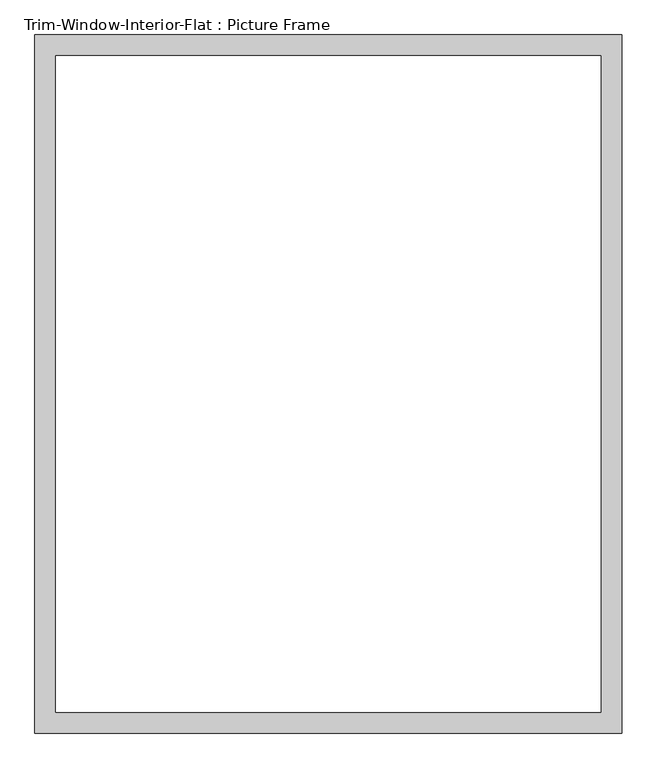
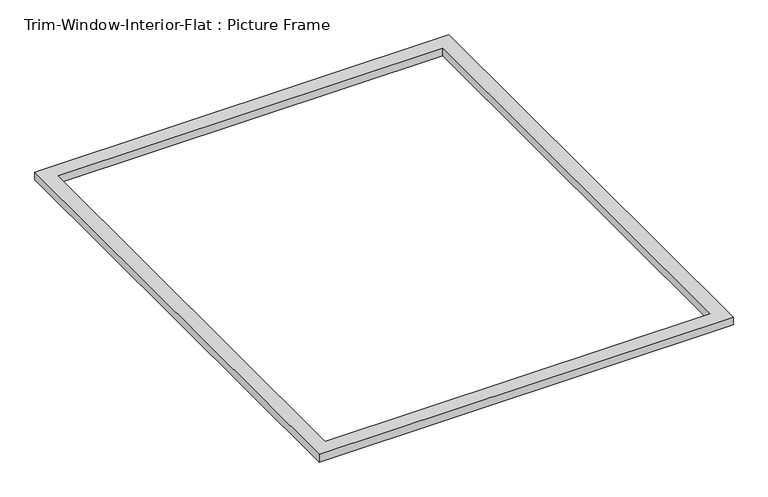
"""IFC4 building model written with IfcOpenShell, lengths in millimetres: proxy geometry, Trim-Window-Interior-Flat : Picture Frame."""

from ifc_helpers import new_model, si_unit, origin, origin_with_axes, place, context, project, spatial, polyline, outline, extrude, source, transform, mapped, element, save


def trim_window_interior_flat_picture_frame_92551a5e(model_context):
    return source(origin(), model_context, "Body", "SweptSolid", [
        extrude(outline(polyline([(806.45, 44.45), (806.45, -1873.25), (-806.45, -1873.25), (-806.45, 44.45), (806.45, 44.45)]), holes=[polyline([(749.3, -12.7), (-749.3, -12.7), (-749.3, -1816.1), (749.3, -1816.1), (749.3, -12.7)])]), origin_with_axes(), (0.0, 0.0, 1.0), 31.75),
    ])


if __name__ == "__main__":
    model = new_model("IFC4")
    model_context = context("Model", 3, world=origin())
    ifc_project = project(units=[si_unit("LENGTHUNIT", "METRE", prefix="MILLI")], contexts=[model_context])
    site = spatial("IfcSite", under=ifc_project)
    building = spatial("IfcBuilding", under=site)
    placement = place(None, origin())
    trim_window_interior_flat_picture_frame_shape = trim_window_interior_flat_picture_frame_92551a5e(model_context)
    element("IfcBuildingElementProxy", 1, Name="Trim-Window-Interior-Flat : Picture Frame", ObjectType="Trim-Window-Interior-Flat : Picture Frame", at=placement, inside=building, context=model_context, shape_type="MappedRepresentation", body=[
        mapped(trim_window_interior_flat_picture_frame_shape, transform((0.0, 0.0, 0.0), x_axis=(1.0, 0.0, 0.0), y_axis=(0.0, 1.0, 0.0), z_axis=(0.0, 0.0, 1.0))),
    ])
    save(model, "model.ifc")

# Revit data of these elements
# Type "Trim-Window-Interior-Flat : Picture Frame"
#   Trim Thickness_Picture Frame = 0' - 1 1/4"
#   Trim Width = 0' - 2 1/4"
#   Trim Thickness_with Sill = 0' - 0 3/4"
#   Sill Thickness = 0' - 1 1/4"
#   Opening Width [instance default] = 2' - 0"
#   Opening Height [instance default] = 3' - 0"
#   Default Elevation = 4' - 0"
#   Sill = no
#   Picture Frame = yes
#   Trim Material [instance default] = none
# Element 1 (IfcBuildingElementProxy, "Trim-Window-Interior-Flat : Picture Frame")
#   Opening Width = 5' - 0"
#   Opening Height = 6' - 0"
#   Trim Material = Wood - Stained
#   Materials on its faces: "Wood - Stained"
# Materials
#   "Wood - Stained": class "Wood", colour RGB 224 178 126, transparency 0, Cost = 0
